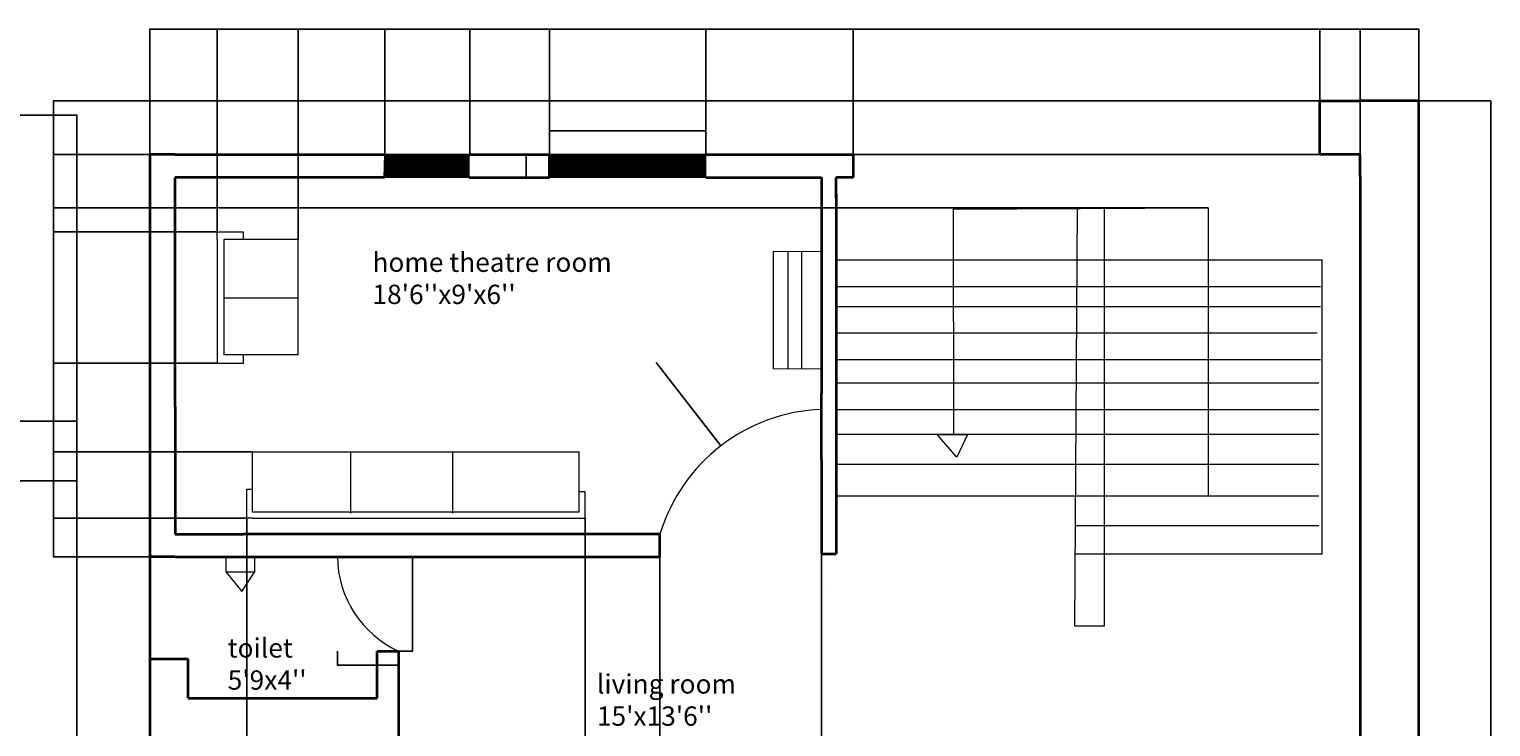
# Model space of a CAD drawing. Units: millimetres. Extents: x 1942 to 12281, y -2698 to 3078.
# Tile 6 of 6: x 6981 to 12281, y 547 to 3078. Entities that reach past the tile are written whole.
import ezdxf

# ---------------------------------------------------------------- set-up
doc = ezdxf.new("R2010")
doc.units = ezdxf.units.MM
for name, color, linetype, lineweight in [('A-ANNO-DIMS', 2, 'Continuous', 18), ('A-AREA-IDEN', 3, 'Continuous', 18), ('A-DOOR', 4, 'Continuous', 18), ('A-EQPM', 8, 'Continuous', 18), ('A-FLOR-FIXT', 9, 'Continuous', 18), ('A-FLOR-STRS', 7, 'Continuous', 18), ('A-FURN', 8, 'Continuous', 18), ('A-GLAZ', 4, 'Continuous', 18), ('A-GLAZ-PATT', 9, 'Continuous', 13), ('A-WALL', 7, 'Continuous', 35)]:
    doc.layers.add(name, color=color, linetype=linetype, lineweight=lineweight)
doc.styles.get("Standard").update_dxf_attribs({"font": 'arial.ttf'})
doc.dimstyles.get("Standard").update_dxf_attribs({"dimtxt": 0.18, "dimasz": 0.18, "dimexe": 0.18, "dimexo": 0.0625, "dimgap": 0.09, "dimtad": 0, "dimtih": 1, "dimtoh": 1, "dimdec": 4, "dimzin": 0, "dimdsep": 46, "dimtxsty": 'Standard', "dimcen": 0.09, "dimadec": 0, "dimazin": 0, "dimtfac": 1, "dimtdec": 4, "dimtofl": 0, "dimtmove": 0, "dimatfit": 3, "dimfxl": 1, "dimtolj": 1, "dimtzin": 0, "dimarcsym": 0})

# ---------------------------------------------------------------- blocks, each defined once
blk = doc.blocks.new('STAIR-RETURN')
for p, q in [((423.4, 1512.5), (1348.3, 1516.9)), ((423.4, 1512.5), (425.2, 695.6)), ((873.7, 1514.6), (863.4, 0)), ((972, 0), (972, 1515.1)), ((1348.3, 1516.9), (1348.3, 695.6)), ((0, 1328.6), (1761.6, 1328.6)), ((1761.6, 261.6), (1761.6, 1328.6)), ((0, 1232.1), (1755.6, 1232.1)), ((0, 1159.8), (1755.6, 1159.8)), ((0, 1063.3), (1743.5, 1063.3)), ((0, 966.9), (1755.6, 966.9)), ((0, 882.5), (1749.6, 882.5)), ((0, 786.1), (1749.6, 786.1)), ((0, 695.6), (1749.6, 695.6)), ((365.9, 694.8), (476.3, 694.8)), ((365.9, 694.8), (476.3, 694.8)), ((365.9, 694.8), (476.3, 694.8)), ((365.9, 694.8), (476.3, 694.8)), ((365.9, 694.8), (476.3, 694.8)), ((365.9, 694.8), (476.3, 694.8)), ((437.5, 612.8), (365.9, 694.8)), ((365.9, 694.8), (476.3, 694.8)), ((476.3, 694.8), (437.5, 612.8)), ((1348.3, 695.6), (1348.3, 587.1)), ((0, 587.1), (1749.6, 587.1)), ((1348.3, 587.1), (1348.3, 472.6)), ((0, 472.6), (1749.6, 472.6)), ((865.9, 364.1), (1749.6, 364.1)), ((865.2, 261.6), (1761.6, 261.6)), ((863.4, 0), (972, 0))]:
    blk.add_line(p, q)
blk = doc.blocks.new('WC-TAPERED')
for p, q in [((0, 69.7), (57.2, 0)), ((57.2, 0), (103.2, 69.7))]:
    blk.add_line(p, q)
blk.add_lwpolyline([(0, 126.7), (103.2, 126.7), (103.2, 69.7), (0, 69.7)], close=True)
blk = doc.blocks.new('DOOR-WC-LIVING')
blk.add_arc((380.4, 345.6), 380.4, 180.4328, 245.2749)
blk = doc.blocks.new('WIN-308')
for p, q in [((2.1, 83.8), (2.1, 0)), ((2.1, 83.8), (310.4, 83.8)), ((310.4, 83.8), (308.2, 0.3)), ((0, 0.3), (308.2, 0.3))]:
    blk.add_line(p, q)
blk = doc.blocks.new('WIN-567')
for p, q in [((0, 83.5), (0, 0)), ((0, 83.5), (567, 83.5)), ((567, 83.5), (567, 0)), ((567, 0), (0, 0))]:
    blk.add_line(p, q)
blk = doc.blocks.new('*D42')
at = {"layer": 'A-ANNO-DIMS', "color": 0, "lineweight": -2, "transparency": 16777216}
for p, q in [((8320.3, 1163.8), (8371.8, 1163.8)), ((8371.6, 1163.6), (8371.6, 992.6)), ((8371.6, 821.3), (8371.6, 992.3)), ((8320.3, 821.1), (8371.8, 821.1))]:
    blk.add_line(p, q, dxfattribs=at)
at = {"layer": 'A-ANNO-DIMS', "color": 0, "transparency": 16777216}
for points in [[(8371.6, 1163.6), (8371.7, 1163.6), (8371.6, 1163.8)], [(8371.6, 821.3), (8371.7, 821.3), (8371.6, 821.1)]]:
    blk.add_solid(points, dxfattribs=at)
at = {"layer": 'Defpoints', "color": 0, "transparency": 16777216}
for p in [(8320.2, 1163.8), (8371.6, 1163.8), (8320.2, 821.1)]:
    blk.add_point(p, dxfattribs=at)
at = {"layer": 'A-ANNO-DIMS', "color": 0, "transparency": 16777216, "insert": (8371.6, 992.5), "char_height": 0.18, "attachment_point": 5}
blk.add_mtext('\\A1;WC DOOR 343 TYP.', dxfattribs=at)
blk = doc.blocks.new('*D43')
at = {"layer": 'A-ANNO-DIMS', "color": 0, "lineweight": -2, "transparency": 16777216}
for p, q in [((8098.9, 821), (8098.9, 769.5)), ((8320.2, 821), (8320.2, 769.5)), ((8099.1, 769.7), (8209, 769.7)), ((8320.1, 769.7), (8210.2, 769.7))]:
    blk.add_line(p, q, dxfattribs=at)
at = {"layer": 'A-ANNO-DIMS', "color": 0, "transparency": 16777216}
for points in [[(8099.1, 769.7), (8099.1, 769.7), (8098.9, 769.7)], [(8320.1, 769.7), (8320.1, 769.7), (8320.2, 769.7)]]:
    blk.add_solid(points, dxfattribs=at)
at = {"layer": 'Defpoints', "color": 0, "transparency": 16777216}
for p in [(8098.9, 821.1), (8320.2, 821.1), (8320.2, 769.7)]:
    blk.add_point(p, dxfattribs=at)
at = {"layer": 'A-ANNO-DIMS', "color": 0, "transparency": 16777216, "insert": (8209.6, 769.7), "char_height": 0.18, "attachment_point": 5}
blk.add_mtext('\\A1;221 TYP.', dxfattribs=at)
blk = doc.blocks.new('*D62')
at = {"layer": 'A-ANNO-DIMS', "color": 0, "lineweight": -2, "transparency": 16777216}
for p, q in [((8867.9, 2623.8), (8867.9, 2708.9)), ((8868, 2708.8), (9150.5, 2708.8)), ((9434.7, 2708.8), (9152.2, 2708.8)), ((9434.8, 2623.8), (9434.8, 2708.9))]:
    blk.add_line(p, q, dxfattribs=at)
at = {"layer": 'A-ANNO-DIMS', "color": 0, "transparency": 16777216}
for points in [[(8868, 2708.8), (8868, 2708.7), (8867.9, 2708.8)], [(9434.7, 2708.8), (9434.7, 2708.7), (9434.8, 2708.8)]]:
    blk.add_solid(points, dxfattribs=at)
at = {"layer": 'Defpoints', "color": 0, "transparency": 16777216}
for p in [(8867.9, 2708.8), (8867.9, 2623.7), (9434.8, 2623.7)]:
    blk.add_point(p, dxfattribs=at)
at = {"layer": 'A-ANNO-DIMS', "color": 0, "transparency": 16777216, "insert": (9151.4, 2708.8), "char_height": 0.18, "attachment_point": 5}
blk.add_mtext('\\A1;W2 567 TYP.', dxfattribs=at)
blk = doc.blocks.new('*D63')
at = {"layer": 'A-ANNO-DIMS', "color": 0, "lineweight": -2, "transparency": 16777216}
for p, q in [((8867.8, 2623.7), (8782.6, 2623.7)), ((8782.8, 2623.5), (8782.8, 2582.1)), ((8782.8, 2540.4), (8782.8, 2581.8)), ((8867.8, 2540.2), (8782.6, 2540.2))]:
    blk.add_line(p, q, dxfattribs=at)
at = {"layer": 'A-ANNO-DIMS', "color": 0, "transparency": 16777216}
for points in [[(8782.8, 2623.5), (8782.9, 2623.5), (8782.8, 2623.7)], [(8782.8, 2540.4), (8782.9, 2540.4), (8782.8, 2540.2)]]:
    blk.add_solid(points, dxfattribs=at)
at = {"layer": 'Defpoints', "color": 0, "transparency": 16777216}
for p in [(8867.9, 2623.7), (8782.8, 2540.2), (8867.9, 2540.2)]:
    blk.add_point(p, dxfattribs=at)
at = {"layer": 'A-ANNO-DIMS', "color": 0, "transparency": 16777216, "insert": (8782.8, 2581.9), "char_height": 0.18, "attachment_point": 5}
blk.add_mtext('\\A1;84 TYP.', dxfattribs=at)
blk = doc.blocks.new('*D71')
at = {"layer": 'A-ANNO-DIMS', "color": 0, "lineweight": -2, "transparency": 16777216}
for p, q in [((6894.2, 2765.9), (7154.5, 2765.9)), ((7154.3, 2765.7), (7154.3, 164.5)), ((7154.3, -2437.1), (7154.3, 164.1)), ((6894.2, -2437.2), (7154.5, -2437.2))]:
    blk.add_line(p, q, dxfattribs=at)
at = {"layer": 'A-ANNO-DIMS', "color": 0, "transparency": 16777216}
for points in [[(7154.3, 2765.7), (7154.4, 2765.7), (7154.3, 2765.9)], [(7154.3, -2437.1), (7154.4, -2437.1), (7154.3, -2437.2)]]:
    blk.add_solid(points, dxfattribs=at)
at = {"layer": 'Defpoints', "color": 0, "transparency": 16777216}
for p in [(6894.1, 2765.9), (7154.3, 2765.9), (6894.1, -2437.2)]:
    blk.add_point(p, dxfattribs=at)
at = {"layer": 'A-ANNO-DIMS', "color": 0, "transparency": 16777216, "insert": (7154.3, 164.3), "char_height": 0.18, "attachment_point": 5}
blk.add_mtext('\\A1;5203', dxfattribs=at)
blk = doc.blocks.new('*D86')
at = {"layer": 'A-ANNO-DIMS', "color": 0, "lineweight": -2, "transparency": 16777216}
for p, q in [((2750.6, 1655.8), (7154.5, 1655.8)), ((7154.3, 1655.6), (7154.3, 1547.7)), ((7154.3, 1439.4), (7154.3, 1547.3)), ((2750.6, 1439.2), (7154.5, 1439.2))]:
    blk.add_line(p, q, dxfattribs=at)
at = {"layer": 'A-ANNO-DIMS', "color": 0, "transparency": 16777216}
for points in [[(7154.3, 1655.6), (7154.4, 1655.6), (7154.3, 1655.8)], [(7154.3, 1439.4), (7154.4, 1439.4), (7154.3, 1439.2)]]:
    blk.add_solid(points, dxfattribs=at)
at = {"layer": 'Defpoints', "color": 0, "transparency": 16777216}
for p in [(2750.5, 1655.8), (7154.3, 1655.8), (2750.5, 1439.2)]:
    blk.add_point(p, dxfattribs=at)
at = {"layer": 'A-ANNO-DIMS', "color": 0, "transparency": 16777216, "insert": (7154.3, 1547.5), "char_height": 0.18, "attachment_point": 5}
blk.add_mtext('\\A1;216.57', dxfattribs=at)
blk = doc.blocks.new('*D92')
at = {"layer": 'A-ANNO-DIMS', "color": 0, "lineweight": -2, "transparency": 16777216}
for p, q in [((7418.5, 2623.8), (7418.5, 3078)), ((7418.7, 3077.8), (9719.2, 3077.8)), ((12020.4, 3077.8), (9719.9, 3077.8)), ((12020.6, 2817.7), (12020.6, 3078))]:
    blk.add_line(p, q, dxfattribs=at)
at = {"layer": 'A-ANNO-DIMS', "color": 0, "transparency": 16777216}
for points in [[(7418.7, 3077.8), (7418.7, 3077.8), (7418.5, 3077.8)], [(12020.4, 3077.8), (12020.4, 3077.8), (12020.6, 3077.8)]]:
    blk.add_solid(points, dxfattribs=at)
at = {"layer": 'Defpoints', "color": 0, "transparency": 16777216}
for p in [(12020.6, 3077.8), (12020.6, 2817.6), (7418.5, 2623.7)]:
    blk.add_point(p, dxfattribs=at)
at = {"layer": 'A-ANNO-DIMS', "color": 0, "transparency": 16777216, "insert": (9719.6, 3077.8), "char_height": 0.18, "attachment_point": 5}
blk.add_mtext('\\A1;4602', dxfattribs=at)
blk = doc.blocks.new('*D93')
at = {"layer": 'A-ANNO-DIMS', "color": 0, "lineweight": -2, "transparency": 16777216}
for p, q in [((12020.6, 2817.6), (12281, 2817.6)), ((12280.8, 2817.4), (12280.8, 216.2)), ((12280.8, -2385.3), (12280.8, 215.9)), ((12020.6, -2385.5), (12281, -2385.5))]:
    blk.add_line(p, q, dxfattribs=at)
at = {"layer": 'A-ANNO-DIMS', "color": 0, "transparency": 16777216}
for points in [[(12280.7, 2817.4), (12280.8, 2817.4), (12280.8, 2817.6)], [(12280.7, -2385.3), (12280.8, -2385.3), (12280.8, -2385.5)]]:
    blk.add_solid(points, dxfattribs=at)
at = {"layer": 'Defpoints', "color": 0, "transparency": 16777216}
for p in [(12020.6, 2817.6), (12280.8, 2817.6), (12020.6, -2385.5)]:
    blk.add_point(p, dxfattribs=at)
at = {"layer": 'A-ANNO-DIMS', "color": 0, "transparency": 16777216, "insert": (12280.8, 216.1), "char_height": 0.18, "attachment_point": 5}
blk.add_mtext('\\A1;5203', dxfattribs=at)
blk = doc.blocks.new('*D94')
at = {"layer": 'A-ANNO-DIMS', "color": 0, "lineweight": -2, "transparency": 16777216}
for p, q in [((7418.5, 2623.7), (7068.5, 2623.7)), ((7068.7, 2623.5), (7068.7, 1893.9)), ((7068.7, 1164), (7068.7, 1893.6)), ((7418.5, 1163.8), (7068.5, 1163.8))]:
    blk.add_line(p, q, dxfattribs=at)
at = {"layer": 'A-ANNO-DIMS', "color": 0, "transparency": 16777216}
for points in [[(7068.7, 2623.5), (7068.8, 2623.5), (7068.7, 2623.7)], [(7068.7, 1164), (7068.8, 1164), (7068.7, 1163.8)]]:
    blk.add_solid(points, dxfattribs=at)
at = {"layer": 'Defpoints', "color": 0, "transparency": 16777216}
for p in [(7068.7, 2623.7), (7418.5, 2623.7), (7418.5, 1163.8)]:
    blk.add_point(p, dxfattribs=at)
at = {"layer": 'A-ANNO-DIMS', "color": 0, "transparency": 16777216, "insert": (7068.7, 1893.8), "char_height": 0.18, "attachment_point": 5}
blk.add_mtext('\\A1;1460', dxfattribs=at)
blk = doc.blocks.new('*D100')
at = {"layer": 'A-ANNO-DIMS', "color": 0, "lineweight": -2, "transparency": 16777216}
for p, q in [((7418.5, 2623.8), (7418.5, 3078)), ((7418.7, 3077.8), (7844, 3077.8)), ((8270.1, 3077.8), (7844.8, 3077.8)), ((8270.3, 2623.8), (8270.3, 3078))]:
    blk.add_line(p, q, dxfattribs=at)
at = {"layer": 'A-ANNO-DIMS', "color": 0, "transparency": 16777216}
for points in [[(7418.7, 3077.8), (7418.7, 3077.8), (7418.5, 3077.8)], [(8270.1, 3077.8), (8270.1, 3077.8), (8270.3, 3077.8)]]:
    blk.add_solid(points, dxfattribs=at)
at = {"layer": 'Defpoints', "color": 0, "transparency": 16777216}
for p in [(8270.3, 3077.8), (7418.5, 2623.7), (8270.3, 2623.7)]:
    blk.add_point(p, dxfattribs=at)
at = {"layer": 'A-ANNO-DIMS', "color": 0, "transparency": 16777216, "insert": (7844.4, 3077.8), "char_height": 0.18, "attachment_point": 5}
blk.add_mtext('\\A1;851.7', dxfattribs=at)
blk = doc.blocks.new('*D101')
at = {"layer": 'A-ANNO-DIMS', "color": 0, "lineweight": -2, "transparency": 16777216}
for p, q in [((8579, 2623.9), (8579, 3078)), ((8579.2, 3077.8), (8723, 3077.8)), ((8867.7, 3077.8), (8723.8, 3077.8)), ((8867.9, 2623.8), (8867.9, 3078))]:
    blk.add_line(p, q, dxfattribs=at)
at = {"layer": 'A-ANNO-DIMS', "color": 0, "transparency": 16777216}
for points in [[(8579.2, 3077.8), (8579.2, 3077.8), (8579, 3077.8)], [(8867.7, 3077.8), (8867.7, 3077.8), (8867.9, 3077.8)]]:
    blk.add_solid(points, dxfattribs=at)
at = {"layer": 'Defpoints', "color": 0, "transparency": 16777216}
for p in [(8867.9, 3077.8), (8579, 2623.8), (8867.9, 2623.7)]:
    blk.add_point(p, dxfattribs=at)
at = {"layer": 'A-ANNO-DIMS', "color": 0, "transparency": 16777216, "insert": (8723.4, 3077.8), "char_height": 0.18, "attachment_point": 5}
blk.add_mtext('\\A1;288.9', dxfattribs=at)
blk = doc.blocks.new('*D102')
at = {"layer": 'A-ANNO-DIMS', "color": 0, "lineweight": -2, "transparency": 16777216}
for p, q in [((9434.8, 2623.8), (9434.8, 3078)), ((9435, 3077.8), (9701.6, 3077.8)), ((9968.9, 3077.8), (9702.4, 3077.8)), ((9969.1, 2623.8), (9969.1, 3078))]:
    blk.add_line(p, q, dxfattribs=at)
at = {"layer": 'A-ANNO-DIMS', "color": 0, "transparency": 16777216}
for points in [[(9435, 3077.8), (9435, 3077.8), (9434.8, 3077.8)], [(9968.9, 3077.8), (9968.9, 3077.8), (9969.1, 3077.8)]]:
    blk.add_solid(points, dxfattribs=at)
at = {"layer": 'Defpoints', "color": 0, "transparency": 16777216}
for p in [(9969.1, 3077.8), (9434.8, 2623.7), (9969.1, 2623.7)]:
    blk.add_point(p, dxfattribs=at)
at = {"layer": 'A-ANNO-DIMS', "color": 0, "transparency": 16777216, "insert": (9702, 3077.8), "char_height": 0.18, "attachment_point": 5}
blk.add_mtext('\\A1;534.2', dxfattribs=at)
blk = doc.blocks.new('*D105')
at = {"layer": 'A-ANNO-DIMS', "color": 0, "lineweight": -2, "transparency": 16777216}
for p, q in [((7769.8, 1304.1), (7769.8, -2645.9)), ((8996.6, 1304.1), (8996.6, -2645.9)), ((7770, -2645.7), (8382.7, -2645.7)), ((8996.4, -2645.7), (8383.6, -2645.7))]:
    blk.add_line(p, q, dxfattribs=at)
at = {"layer": 'A-ANNO-DIMS', "color": 0, "transparency": 16777216}
for points in [[(7770, -2645.7), (7770, -2645.7), (7769.8, -2645.7)], [(8996.4, -2645.7), (8996.4, -2645.7), (8996.6, -2645.7)]]:
    blk.add_solid(points, dxfattribs=at)
at = {"layer": 'Defpoints', "color": 0, "transparency": 16777216}
for p in [(7769.8, 1304.1), (8996.6, 1304.1), (8996.6, -2645.7)]:
    blk.add_point(p, dxfattribs=at)
at = {"layer": 'A-ANNO-DIMS', "color": 0, "transparency": 16777216, "insert": (8383.2, -2645.7), "char_height": 0.18, "attachment_point": 5}
blk.add_mtext('\\A1;1226.8', dxfattribs=at)
blk = doc.blocks.new('*D106')
at = {"layer": 'A-ANNO-DIMS', "color": 0, "lineweight": -2, "transparency": 16777216}
for p, q in [((7790, 1544.9), (7068.5, 1544.9)), ((7068.7, 1544.7), (7068.7, 1424.7)), ((7068.7, 1304.3), (7068.7, 1424.3)), ((7769.7, 1304.1), (7068.5, 1304.1))]:
    blk.add_line(p, q, dxfattribs=at)
at = {"layer": 'A-ANNO-DIMS', "color": 0, "transparency": 16777216}
for points in [[(7068.7, 1544.7), (7068.8, 1544.7), (7068.7, 1544.9)], [(7068.7, 1304.3), (7068.8, 1304.3), (7068.7, 1304.1)]]:
    blk.add_solid(points, dxfattribs=at)
at = {"layer": 'Defpoints', "color": 0, "transparency": 16777216}
for p in [(7068.7, 1544.9), (7790.1, 1544.9), (7769.8, 1304.1)]:
    blk.add_point(p, dxfattribs=at)
at = {"layer": 'A-ANNO-DIMS', "color": 0, "transparency": 16777216, "insert": (7068.7, 1424.5), "char_height": 0.18, "attachment_point": 5}
blk.add_mtext('\\A1;240.74', dxfattribs=at)
blk = doc.blocks.new('*D107')
at = {"layer": 'A-ANNO-DIMS', "color": 0, "lineweight": -2, "transparency": 16777216}
for p, q in [((7662.5, 2343.2), (7662.5, 3078)), ((7662.7, 3077.8), (7809, 3077.8)), ((7956.1, 3077.8), (7809.8, 3077.8)), ((7956.3, 2314.7), (7956.3, 3078))]:
    blk.add_line(p, q, dxfattribs=at)
at = {"layer": 'A-ANNO-DIMS', "color": 0, "transparency": 16777216}
for points in [[(7662.7, 3077.8), (7662.7, 3077.8), (7662.5, 3077.8)], [(7956.1, 3077.8), (7956.1, 3077.8), (7956.3, 3077.8)]]:
    blk.add_solid(points, dxfattribs=at)
at = {"layer": 'Defpoints', "color": 0, "transparency": 16777216}
for p in [(7956.3, 3077.8), (7662.5, 2343.1), (7956.3, 2314.6)]:
    blk.add_point(p, dxfattribs=at)
at = {"layer": 'A-ANNO-DIMS', "color": 0, "transparency": 16777216, "insert": (7809.4, 3077.8), "char_height": 0.18, "attachment_point": 5}
blk.add_mtext('\\A1;293.8', dxfattribs=at)
blk = doc.blocks.new('*D108')
at = {"layer": 'A-ANNO-DIMS', "color": 0, "lineweight": -2, "transparency": 16777216}
for p, q in [((7662.4, 2343.1), (7068.5, 2343.1)), ((7068.7, 2342.9), (7068.7, 2104.9)), ((7068.7, 1866.5), (7068.7, 2104.5)), ((7662.4, 1866.3), (7068.5, 1866.3))]:
    blk.add_line(p, q, dxfattribs=at)
at = {"layer": 'A-ANNO-DIMS', "color": 0, "transparency": 16777216}
for points in [[(7068.7, 2342.9), (7068.8, 2342.9), (7068.7, 2343.1)], [(7068.7, 1866.5), (7068.8, 1866.5), (7068.7, 1866.3)]]:
    blk.add_solid(points, dxfattribs=at)
at = {"layer": 'Defpoints', "color": 0, "transparency": 16777216}
for p in [(7068.7, 2343.1), (7662.5, 2343.1), (7662.5, 1866.3)]:
    blk.add_point(p, dxfattribs=at)
at = {"layer": 'A-ANNO-DIMS', "color": 0, "transparency": 16777216, "insert": (7068.7, 2104.7), "char_height": 0.18, "attachment_point": 5}
blk.add_mtext('\\A1;476.8', dxfattribs=at)
blk = doc.blocks.new('*D109')
at = {"layer": 'A-ANNO-DIMS', "color": 0, "lineweight": -2, "transparency": 16777216}
for p, q in [((9268.3, 1245.3), (9268.3, -2645.9)), ((9854.3, 1173.9), (9854.3, -2645.9)), ((9268.4, -2645.7), (9561, -2645.7)), ((9854.1, -2645.7), (9561.5, -2645.7))]:
    blk.add_line(p, q, dxfattribs=at)
at = {"layer": 'A-ANNO-DIMS', "color": 0, "transparency": 16777216}
for points in [[(9268.4, -2645.7), (9268.4, -2645.7), (9268.3, -2645.7)], [(9854.1, -2645.7), (9854.1, -2645.7), (9854.3, -2645.7)]]:
    blk.add_solid(points, dxfattribs=at)
at = {"layer": 'Defpoints', "color": 0, "transparency": 16777216}
for p in [(9268.3, 1245.4), (9854.3, 1174), (9854.3, -2645.7)]:
    blk.add_point(p, dxfattribs=at)
at = {"layer": 'A-ANNO-DIMS', "color": 0, "transparency": 16777216, "insert": (9561.3, -2645.7), "char_height": 0.18, "attachment_point": 5}
blk.add_mtext('\\A1;586', dxfattribs=at)
blk = doc.blocks.new('*D110')
at = {"layer": 'A-ANNO-DIMS', "color": 0, "lineweight": -2, "transparency": 16777216}
for p, q in [((11661, 2817.6), (7068.5, 2817.6)), ((7068.7, 2817.4), (7068.7, 2720.8)), ((7068.7, 2623.9), (7068.7, 2720.5)), ((11661, 2623.7), (7068.5, 2623.7))]:
    blk.add_line(p, q, dxfattribs=at)
at = {"layer": 'A-ANNO-DIMS', "color": 0, "transparency": 16777216}
for points in [[(7068.7, 2817.4), (7068.8, 2817.4), (7068.7, 2817.6)], [(7068.7, 2623.9), (7068.8, 2623.9), (7068.7, 2623.7)]]:
    blk.add_solid(points, dxfattribs=at)
at = {"layer": 'Defpoints', "color": 0, "transparency": 16777216}
for p in [(7068.7, 2817.6), (11661, 2817.6), (11661, 2623.7)]:
    blk.add_point(p, dxfattribs=at)
at = {"layer": 'A-ANNO-DIMS', "color": 0, "transparency": 16777216, "insert": (7068.7, 2720.7), "char_height": 0.18, "attachment_point": 5}
blk.add_mtext('\\A1;193.9', dxfattribs=at)
blk = doc.blocks.new('*D111')
at = {"layer": 'A-ANNO-DIMS', "color": 0, "lineweight": -2, "transparency": 16777216}
for p, q in [((11661, 2623.8), (11661, 3078)), ((11661.2, 3077.8), (11734.1, 3077.8)), ((11807.8, 3077.8), (11734.9, 3077.8)), ((11807.9, 2623.8), (11807.9, 3078))]:
    blk.add_line(p, q, dxfattribs=at)
at = {"layer": 'A-ANNO-DIMS', "color": 0, "transparency": 16777216}
for points in [[(11661.2, 3077.8), (11661.2, 3077.8), (11661, 3077.8)], [(11807.8, 3077.8), (11807.8, 3077.8), (11807.9, 3077.8)]]:
    blk.add_solid(points, dxfattribs=at)
at = {"layer": 'Defpoints', "color": 0, "transparency": 16777216}
for p in [(11807.9, 3077.8), (11661, 2623.7), (11807.9, 2623.7)]:
    blk.add_point(p, dxfattribs=at)
at = {"layer": 'A-ANNO-DIMS', "color": 0, "transparency": 16777216, "insert": (11734.5, 3077.8), "char_height": 0.18, "attachment_point": 5}
blk.add_mtext('\\A1;146.9', dxfattribs=at)
blk = doc.blocks.new('*D112')
at = {"layer": 'A-ANNO-DIMS', "color": 0, "lineweight": -2, "transparency": 16777216}
for p, q in [((11661, 2623.7), (7068.5, 2623.7)), ((7068.7, 2623.5), (7068.7, 2526.6)), ((7068.7, 2429.4), (7068.7, 2526.3)), ((11256, 2429.2), (7068.5, 2429.2))]:
    blk.add_line(p, q, dxfattribs=at)
at = {"layer": 'A-ANNO-DIMS', "color": 0, "transparency": 16777216}
for points in [[(7068.7, 2623.5), (7068.8, 2623.5), (7068.7, 2623.7)], [(7068.7, 2429.4), (7068.8, 2429.4), (7068.7, 2429.2)]]:
    blk.add_solid(points, dxfattribs=at)
at = {"layer": 'Defpoints', "color": 0, "transparency": 16777216}
for p in [(7068.7, 2623.7), (11661, 2623.7), (11256.1, 2429.2)]:
    blk.add_point(p, dxfattribs=at)
at = {"layer": 'A-ANNO-DIMS', "color": 0, "transparency": 16777216, "insert": (7068.7, 2526.5), "char_height": 0.18, "attachment_point": 5}
blk.add_mtext('\\A1;194.5', dxfattribs=at)
blk = doc.blocks.new('*D118')
at = {"layer": 'A-ANNO-DIMS', "color": 0, "lineweight": -2, "transparency": 16777216}
for p, q in [((9254.6, 1868.3), (9254.8, 1868.3)), ((9254.8, 1868.3), (9488.6, 1565.9)), ((9878.4, 1061.5), (9878.4, 1061.7)), ((9878.4, 1061.6), (9878.5, 1061.6))]:
    blk.add_line(p, q, dxfattribs=at)
at = {"layer": 'A-ANNO-DIMS', "color": 0, "transparency": 16777216}
blk.add_solid([(9488.6, 1565.9), (9488.5, 1565.9), (9488.7, 1565.8)], dxfattribs=at)
at = {"layer": 'Defpoints', "color": 0, "transparency": 16777216}
for p in [(9488.7, 1565.8), (9878.4, 1061.6)]:
    blk.add_point(p, dxfattribs=at)
at = {"layer": 'A-ANNO-DIMS', "color": 0, "transparency": 16777216, "insert": (9254.2, 1868.3), "char_height": 0.18, "attachment_point": 5}
blk.add_mtext('\\A1;R637.3', dxfattribs=at)

msp = doc.modelspace()

# ---------------------------------------------------------------- hatches: boundary and pattern name
at = {"layer": 'A-GLAZ-PATT'}
h = msp.add_hatch(dxfattribs=at)
h.set_pattern_fill('ANSI31', color=256, scale=1.199911, angle=135, style=0)
h.paths.add_polyline_path([(8270.251, 2539.896), (8576.356, 2540.178), (8578.5, 2623.71), (8270.251, 2623.71)])
h = msp.add_hatch(dxfattribs=at)
h.set_pattern_fill('ANSI31', color=256, scale=1.384708, angle=135, style=0)
h.paths.add_polyline_path([(8867.867, 2540.178), (9434.843, 2540.178), (9434.843, 2623.71), (8867.867, 2623.71)])

# ---------------------------------------------------------------- linework, layer by layer
at = {"layer": 'A-DOOR'}
msp.add_arc((9878.449, 1061.605), 637.261, 92.175374, 163.238996, dxfattribs=at)
at = {"layer": 'A-EQPM'}
for p, q in [((9678.426, 2270.734), (9854.26, 2272.83)), ((9678.426, 2271.97), (9678.426, 1845.56)), ((9731.934, 2271.97), (9731.934, 1845.56)), ((9782.094, 2271.97), (9782.094, 1845.56)), ((9678.426, 1846.297), (9854.26, 1845.048))]:
    msp.add_line(p, q, dxfattribs=at)
at = {"layer": 'A-FURN'}
for p, q in [((7662.506, 2314.611), (7662.506, 2343.09)), ((7662.506, 2343.09), (7756.505, 2343.09)), ((7756.505, 2343.09), (7756.505, 2314.611)), ((7662.506, 2314.611), (7662.506, 2100.619)), ((7662.506, 2312.88), (7662.506, 2100.619)), ((7686.467, 2314.611), (7686.467, 2102.35)), ((7956.299, 2314.611), (7686.467, 2314.611)), ((7956.299, 1896.097), (7956.299, 2314.611)), ((7662.506, 2100.619), (7662.506, 1894.366)), ((7662.506, 2100.619), (7662.506, 1894.366)), ((7953.351, 2102.35), (7686.467, 2102.35)), ((7686.467, 2102.35), (7686.467, 1896.097)), ((7662.506, 1894.366), (7662.506, 1866.33)), ((7662.506, 1866.33), (7757.611, 1866.33)), ((7958.103, 1896.097), (7686.467, 1896.097)), ((7757.611, 1866.33), (7757.611, 1896.097)), ((7790.05, 1544.871), (8974.807, 1544.871)), ((7790.05, 1544.871), (7790.05, 1326.317)), ((8146.141, 1540.466), (8146.141, 1321.911)), ((8515.502, 1540.466), (8515.502, 1321.911)), ((8974.807, 1326.317), (8974.807, 1544.871)), ((7769.776, 1304.131), (7769.776, 1409.396)), ((7769.776, 1409.396), (7790.05, 1409.396)), ((8996.556, 1399.64), (8974.807, 1399.271)), ((8996.556, 1304.131), (8996.556, 1399.64)), ((7790.05, 1326.317), (8974.807, 1326.317)), ((7790.05, 1304.131), (7769.776, 1304.131)), ((7790.05, 1304.131), (8974.807, 1304.131)), ((8974.807, 1304.131), (8996.556, 1304.131))]:
    msp.add_line(p, q, dxfattribs=at)
at = {"layer": 'A-WALL'}
for p, q in [((11661.033, 2623.71), (11661.033, 2817.617)), ((11661.033, 2817.617), (11804.799, 2817.617)), ((12020.574, 2817.617), (11804.799, 2817.617)), ((12020.574, -434.479), (12020.574, 2817.617)), ((7510.608, 2623.71), (7418.529, 2623.71)), ((7418.529, 2623.71), (7418.529, 1490.955)), ((7510.608, 2623.71), (8270.251, 2623.71)), ((7510.608, 2623.71), (7510.608, 2623.71)), ((8578.5, 2623.71), (8867.867, 2623.71)), ((8867.867, 2540.178), (8867.867, 2623.71)), ((9434.843, 2623.71), (9833.172, 2623.71)), ((9833.172, 2623.71), (9969.072, 2623.71)), ((9969.072, 2623.71), (9969.072, 2540.178)), ((11807.937, 2623.71), (11661.033, 2623.71)), ((11807.937, 2623.71), (11807.937, 2623.71)), ((11807.937, 2543.304), (11807.937, 2623.71)), ((8270.251, 2539.896), (7510.608, 2539.896)), ((7510.608, 1707.522), (7510.608, 2539.896)), ((8576.356, 2540.178), (8867.867, 2540.178)), ((9434.843, 2540.178), (9854.26, 2540.178)), ((9854.26, 2540.178), (9854.26, 2464.641)), ((9907.351, 2464.641), (9907.351, 2540.178)), ((9969.072, 2540.178), (9907.768, 2540.178)), ((11807.937, 2543.304), (11807.937, -434.479)), ((9854.26, 2464.641), (9854.26, 1757.55)), ((9907.351, 2480.89), (9907.768, 2480.888)), ((9907.768, 2480.888), (9907.768, 1515.222)), ((9854.26, 1515.222), (9854.26, 1757.55)), ((7510.608, 1707.522), (7510.608, 1490.955)), ((7418.529, 1490.955), (7418.529, 1163.806)), ((7510.608, 1490.955), (7510.608, 1245.379)), ((9854.26, 1515.222), (9854.26, 1173.953)), ((9907.768, 1515.222), (9907.768, 1173.953)), ((7510.608, 1245.379), (7757.829, 1245.379)), ((7510.608, 1245.379), (7510.608, 1245.379)), ((9268.262, 1245.379), (7757.829, 1245.379)), ((9268.352, 1163.806), (9268.262, 1245.379)), ((9854.26, 1173.953), (9907.768, 1173.953)), ((7418.529, 1163.806), (7418.529, 793.021)), ((7510.608, 1163.806), (7418.529, 1163.806)), ((7510.608, 1163.806), (8867.867, 1163.806)), ((8867.867, 1163.806), (9268.352, 1163.806)), ((8243.328, 650.617), (8243.328, 821.112)), ((8243.328, 821.112), (8320.239, 821.112)), ((8320.239, 821.112), (8320.239, 96.726)), ((7418.529, 793.021), (7557.198, 793.021)), ((7418.529, 793.021), (7418.529, 350.597)), ((7557.198, 650.617), (7557.198, 793.021)), ((7557.198, 650.617), (7777.378, 650.617)), ((7777.378, 650.617), (8091.142, 650.617)), ((8091.142, 650.617), (8243.328, 650.617))]:
    msp.add_line(p, q, dxfattribs=at)

# ---------------------------------------------------------------- block references
at = {"layer": 'A-DOOR'}
msp.add_blockref('DOOR-WC-LIVING', (8098.931, 821.112), dxfattribs=at)
at = {"layer": 'A-FLOR-FIXT'}
msp.add_blockref('WC-TAPERED', (7694.924, 1037.604), dxfattribs=at)
at = {"layer": 'A-FLOR-STRS'}
msp.add_blockref('STAIR-RETURN', (9907.768, 912.356), dxfattribs=at)
at = {"layer": 'A-GLAZ'}
for name, p, rotation in [('WIN-308', (8578.982, 2624.121), 180.0738548572142), ('WIN-567', (9434.842, 2623.71), 180)]:
    msp.add_blockref(name, p, dxfattribs=dict(at, rotation=rotation))

# ---------------------------------------------------------------- texts
at = {"layer": 'A-AREA-IDEN', "char_height": 70, "attachment_point": 1}
for s, insert in [("{home theatre room\\P18'6''x9'x6''}", (8225.764, 2267.407)), ("{toilet\\P5'9x4''}", (7700.843, 867.809)), ("{living room\\P15'x13'6''}", (9039.685, 737.054))]:
    msp.add_mtext(s, dxfattribs=dict(at, insert=insert))

# ---------------------------------------------------------------- dimensions: what is measured, and where the dimension line sits
at = {"layer": 'A-ANNO-DIMS'}
for base, p1, p2, override, picture, middle in [((12020.574, 3077.817), (7418.529, 2623.71), (12020.574, 2817.617), {"dimdec": 0, "dimlfac": 1, "dimrnd": 0, "dimzin": 0, "dimdsep": 46, "dimlunit": 2}, '*D92', (9719.552, 3077.817)), ((8270.251, 3077.817), (7418.529, 2623.71), (8270.251, 2623.71), {"dimdec": 1, "dimlfac": 1, "dimrnd": 0, "dimzin": 0, "dimdsep": 46, "dimlunit": 2}, '*D100', (7844.39, 3077.817)), ((7956.299, 3077.817), (7662.506, 2343.09), (7956.299, 2314.611), {"dimdec": 1, "dimlfac": 1, "dimrnd": 0, "dimzin": 0, "dimdsep": 46, "dimlunit": 2}, '*D107', (7809.403, 3077.817)), ((8867.867, 3077.817), (8578.982, 2623.84), (8867.867, 2623.71), {"dimdec": 1, "dimlfac": 1, "dimrnd": 0, "dimzin": 0, "dimdsep": 46, "dimlunit": 2}, '*D101', (8723.424, 3077.817)), ((9969.072, 3077.817), (9434.843, 2623.71), (9969.072, 2623.71), {"dimdec": 1, "dimlfac": 1, "dimrnd": 0, "dimzin": 0, "dimdsep": 46, "dimlunit": 2}, '*D102', (9701.958, 3077.817)), ((11807.937, 3077.817), (11661.033, 2623.71), (11807.937, 2623.71), {"dimdec": 1, "dimlfac": 1, "dimrnd": 0, "dimzin": 0, "dimdsep": 46, "dimlunit": 2}, '*D111', (11734.485, 3077.817)), ((8996.556, -2645.689), (7769.776, 1304.131), (8996.556, 1304.131), {"dimdec": 1, "dimlfac": 1, "dimrnd": 0, "dimzin": 0, "dimdsep": 46, "dimlunit": 2}, '*D105', (8383.166, -2645.689)), ((9854.26, -2645.689), (9268.262, 1245.379), (9854.26, 1173.953), {"dimdec": 0, "dimlfac": 1, "dimrnd": 0, "dimzin": 0, "dimdsep": 46, "dimlunit": 2}, '*D109', (9561.261, -2645.689))]:
    dim = msp.add_linear_dim(base=base, p1=p1, p2=p2, dimstyle='Standard', override=override, dxfattribs=at)
    dim.commit()
    dim.dimension.update_dxf_attribs({"geometry": picture, "text_midpoint": middle})
for base, p1, p2, override, picture, middle in [((7068.728, 2817.617), (11661.033, 2623.71), (11661.033, 2817.617), {"dimdec": 1, "dimlfac": 1, "dimrnd": 0, "dimzin": 0, "dimdsep": 46, "dimlunit": 2}, '*D110', (7068.728, 2720.664)), ((12280.774, 2817.617), (12020.574, -2385.489), (12020.574, 2817.617), {"dimdec": 0, "dimlfac": 1, "dimrnd": 0, "dimzin": 0, "dimdsep": 46, "dimlunit": 2}, '*D93', (12280.774, 216.064)), ((7154.346, 2765.873), (6894.096, -2437.233), (6894.096, 2765.873), {"dimdec": 0, "dimlfac": 1, "dimrnd": 0, "dimzin": 0, "dimdsep": 46, "dimlunit": 2}, '*D71', (7154.346, 164.32)), ((7068.728, 2623.71), (11256.077, 2429.209), (11661.033, 2623.71), {"dimdec": 1, "dimlfac": 1, "dimrnd": 0, "dimzin": 0, "dimdsep": 46, "dimlunit": 2}, '*D112', (7068.728, 2526.46)), ((7068.728, 2623.71), (7418.529, 1163.806), (7418.529, 2623.71), {"dimdec": 0, "dimlfac": 1, "dimrnd": 0, "dimzin": 0, "dimdsep": 46, "dimlunit": 2}, '*D94', (7068.728, 1893.758)), ((7068.728, 2343.09), (7662.506, 1866.33), (7662.506, 2343.09), {"dimdec": 1, "dimlfac": 1, "dimrnd": 0, "dimzin": 0, "dimdsep": 46, "dimlunit": 2}, '*D108', (7068.728, 2104.71)), ((7154.346, 1655.778), (2750.504, 1439.211), (2750.504, 1655.778), {"dimdec": 2, "dimlfac": 1, "dimrnd": 0, "dimzin": 0, "dimdsep": 46, "dimlunit": 2}, '*D86', (7154.346, 1547.494)), ((7068.728, 1544.871), (7769.776, 1304.131), (7790.05, 1544.871), {"dimdec": 2, "dimlfac": 1, "dimrnd": 0, "dimzin": 0, "dimdsep": 46, "dimlunit": 2}, '*D106', (7068.728, 1424.501))]:
    dim = msp.add_linear_dim(base=base, p1=p1, p2=p2, angle=90, dimstyle='Standard', override=override, dxfattribs=at)
    dim.commit()
    dim.dimension.update_dxf_attribs({"geometry": picture, "text_midpoint": middle})
for base, p1, p2, angle, text, picture, middle in [((8867.867, 2708.757), (9434.843, 2623.71), (8867.867, 2623.71), 180, 'W2 <> TYP.', '*D62', (9151.355, 2708.757)), ((8782.821, 2540.178), (8867.867, 2623.71), (8867.867, 2540.178), 270, '<> TYP.', '*D63', (8782.821, 2581.944)), ((8371.643, 1163.806), (8320.239, 821.112), (8320.239, 1163.806), 90, 'WC DOOR <> TYP.', '*D42', (8371.643, 992.459))]:
    dim = msp.add_linear_dim(base=base, p1=p1, p2=p2, angle=angle, text=text, dimstyle='Standard', override={"dimdec": 0, "dimlfac": 1, "dimrnd": 0, "dimzin": 0, "dimdsep": 46, "dimlunit": 2}, dxfattribs=at)
    dim.commit()
    dim.dimension.update_dxf_attribs({"geometry": picture, "text_midpoint": middle})
dim = msp.add_radius_dim(center=(9878.449, 1061.605), mpoint=(9488.68, 1565.77), dimstyle='Standard', override={"dimdec": 1, "dimlfac": 1, "dimrnd": 0, "dimzin": 0, "dimdsep": 46, "dimlunit": 2}, dxfattribs=at)
dim.commit()
dim.dimension.update_dxf_attribs({"geometry": '*D118', "text_midpoint": (9254.159, 1868.268), "dimtype": 164})
dim = msp.add_linear_dim(base=(8320.239, 769.708), p1=(8098.932, 821.112), p2=(8320.239, 821.112), text='<> TYP.', dimstyle='Standard', override={"dimdec": 0, "dimlfac": 1, "dimrnd": 0, "dimzin": 0, "dimdsep": 46, "dimlunit": 2}, dxfattribs=at)
dim.commit()
dim.dimension.update_dxf_attribs({"geometry": '*D43', "text_midpoint": (8209.585, 769.708)})

doc.saveas('drawing.dxf')
